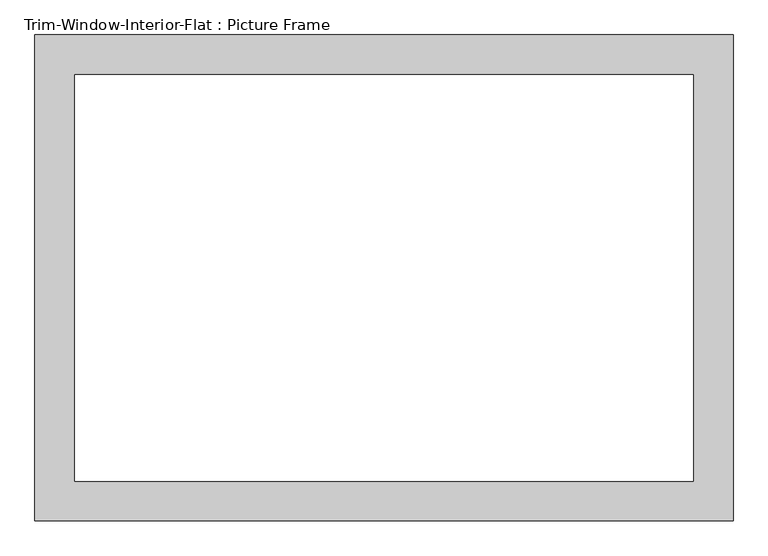
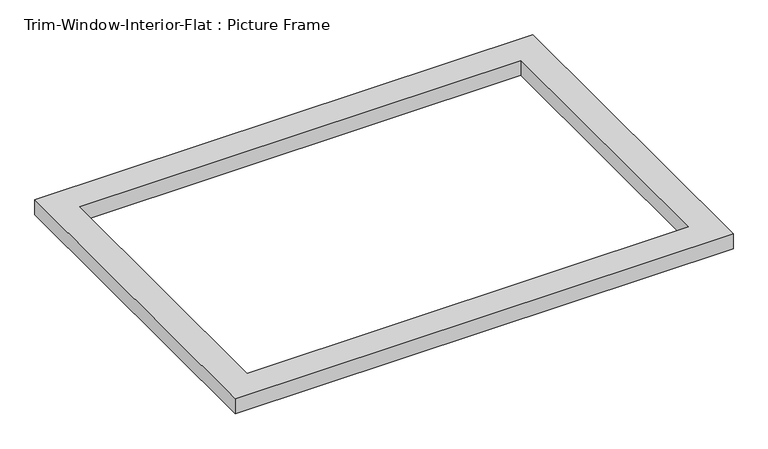
"""IFC4 building model written with IfcOpenShell, lengths in millimetres: proxy geometry, Trim-Window-Interior-Flat : Picture Frame."""

from ifc_helpers import new_model, si_unit, origin, origin_with_axes, place, context, project, spatial, polyline, outline, extrude, source, transform, mapped, element, save


def trim_window_interior_flat_picture_frame_6592d821(model_context):
    return source(origin(), model_context, "Body", "SweptSolid", [
        extrude(outline(polyline([(501.65, 44.45), (501.65, -654.05), (-501.65, -654.05), (-501.65, 44.45), (501.65, 44.45)]), holes=[polyline([(444.5, -12.7), (-444.5, -12.7), (-444.5, -596.9), (444.5, -596.9), (444.5, -12.7)])]), origin_with_axes(), (0.0, 0.0, 1.0), 31.75),
    ])


if __name__ == "__main__":
    model = new_model("IFC4")
    model_context = context("Model", 3, world=origin())
    ifc_project = project(units=[si_unit("LENGTHUNIT", "METRE", prefix="MILLI")], contexts=[model_context])
    site = spatial("IfcSite", under=ifc_project)
    building = spatial("IfcBuilding", under=site)
    placement = place(None, origin())
    trim_window_interior_flat_picture_frame_shape = trim_window_interior_flat_picture_frame_6592d821(model_context)
    element("IfcBuildingElementProxy", 1, Name="Trim-Window-Interior-Flat : Picture Frame", ObjectType="Trim-Window-Interior-Flat : Picture Frame", at=placement, inside=building, context=model_context, shape_type="MappedRepresentation", body=[
        mapped(trim_window_interior_flat_picture_frame_shape, transform((0.0, 0.0, 0.0), x_axis=(1.0, 0.0, 0.0), y_axis=(0.0, 1.0, 0.0), z_axis=(0.0, 0.0, 1.0))),
    ])
    save(model, "model.ifc")

# Revit data of these elements
# Type "Trim-Window-Interior-Flat : Picture Frame"
#   Trim Thickness_Picture Frame = 0' - 1 1/4"
#   Trim Width = 0' - 2 1/4"
#   Trim Thickness_with Sill = 0' - 0 3/4"
#   Sill Thickness = 0' - 1 1/4"
#   Opening Width [instance default] = 2' - 0"
#   Opening Height [instance default] = 3' - 0"
#   Default Elevation = 4' - 0"
#   Sill = no
#   Picture Frame = yes
#   Trim Material [instance default] = none
# Element 1 (IfcBuildingElementProxy, "Trim-Window-Interior-Flat : Picture Frame")
#   Opening Width = 3' - 0"
#   Opening Height = 2' - 0"
#   Trim Material = Wood - Stained
#   Materials on its faces: "Wood - Stained"
# Materials
#   "Wood - Stained": class "Wood", colour RGB 224 178 126, transparency 0, Cost = 0
